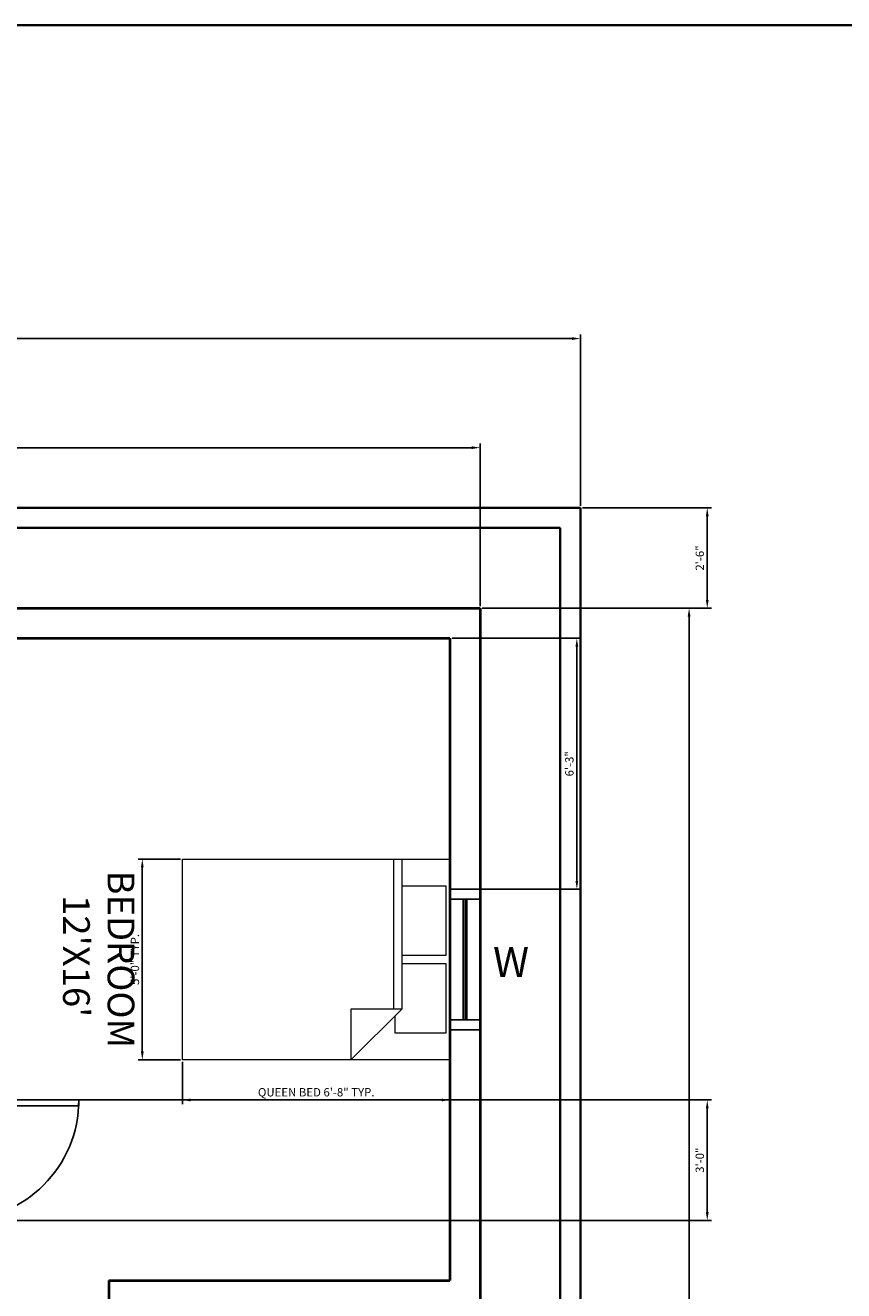
# Model space of a CAD drawing. Units: inches. Extents: x 6038 to 7543, y 3772 to 5131.
# Tile 9 of 14: x 6545 to 6790, y 4753 to 5131. Entities that reach past the tile are written whole.
import ezdxf

# ---------------------------------------------------------------- set-up
doc = ezdxf.new("R2010")
doc.units = ezdxf.units.IN
for name, color, linetype, lineweight in [('A-ANNO-DIMS', 4, 'Continuous', 18), ('A-ANNO-TEXT', 7, 'Continuous', 18), ('A-ANNO-TTLB', 1, 'Continuous', 35), ('A-AREA-IDEN', 2, 'Continuous', 18), ('A-DOOR', 3, 'Continuous', 25), ('A-FURN', 8, 'Continuous', 18), ('A-WALL', 7, 'Continuous', 40)]:
    doc.layers.add(name, color=color, linetype=linetype, lineweight=lineweight)
doc.layers.add('A-GLAZ', color=30, linetype='Continuous', lineweight=25, true_color=0xf26722)
doc.layers.add('C-PROP-WALL', color=251, linetype='Continuous', lineweight=35, true_color=0x636466)
doc.styles.get("Standard").update_dxf_attribs({"font": 'arial.ttf'})
doc.dimstyles.new('ISO-25', dxfattribs={"dimtxt": 2.5, "dimasz": 2.5, "dimexe": 1.25, "dimexo": 0.625, "dimtad": 1, "dimdec": 0, "dimlunit": 3, "dimtxsty": 'Standard', "dimcen": 2.5, "dimadec": 0, "dimazin": 0, "dimtfac": 1, "dimtdec": 0, "dimtmove": 0, "dimatfit": 3, "dimfxl": 1, "dimarcsym": 0})

# ---------------------------------------------------------------- blocks, each defined once
blk = doc.blocks.new('Bed - Queen')
for p, q in [((0, -80.00003), (0, 0)), ((0, 0), (59.99999, 0)), ((59.99999, 0), (59.99999, -80.00003)), ((7.99999, -1.2), (28.79998, -1.2)), ((7.99999, -14.4), (7.99999, -1.2)), ((28.79998, -1.2), (28.79998, -14.4)), ((31.19999, -1.2), (51.99999, -1.2)), ((31.19999, -14.4), (31.19999, -1.2)), ((51.99999, -1.2), (51.99999, -16.4)), ((0, -14.4), (44.8, -14.4)), ((59.99999, -29.6), (44.8, -14.4)), ((44.8, -14.4), (44.8, -29.6)), ((44.8, -16.8), (0, -16.8)), ((51.99999, -16.4), (46.79936, -16.4)), ((44.8, -29.6), (59.99999, -29.6)), ((59.99999, -80.00003), (0, -80.00003))]:
    blk.add_line(p, q)
blk = doc.blocks.new('*U9')
for p, q in [((0, 0), (0, -6)), ((36, 0), (36, -6))]:
    blk.add_line(p, q)
blk.add_lwpolyline([(0, 0), (0, 36), (1.75, 36), (1.75, 0)], close=True)
blk.add_arc((0, 0), 36, 0, 90)
blk = doc.blocks.new('*D13')
at = {"layer": 'A-ANNO-DIMS', "color": 0, "lineweight": -2, "transparency": 16777216}
for p, q in [((6321.42, 4957.24), (6321.42, 5005.85)), ((6323.92, 5004.6), (6678.92, 5004.6)), ((6681.42, 4957.24), (6681.42, 5005.85))]:
    blk.add_line(p, q, dxfattribs=at)
at = {"layer": 'A-ANNO-DIMS', "color": 0, "transparency": 16777216}
for points in [[(6323.92, 5005.02), (6323.92, 5004.19), (6321.42, 5004.6)], [(6678.92, 5005.02), (6678.92, 5004.19), (6681.42, 5004.6)]]:
    blk.add_solid(points, dxfattribs=at)
at = {"layer": 'Defpoints', "color": 0, "transparency": 16777216}
for p in [(6681.42, 5004.6), (6321.42, 4956.62), (6681.42, 4956.62)]:
    blk.add_point(p, dxfattribs=at)
at = {"layer": 'A-ANNO-DIMS', "color": 0, "transparency": 16777216, "insert": (6501.42, 5012.89), "char_height": 2.5, "attachment_point": 5}
blk.add_mtext("{\\H6x;30'}", dxfattribs=at)
blk = doc.blocks.new('*D14')
at = {"layer": 'A-ANNO-DIMS', "color": 0, "lineweight": -2, "transparency": 16777216}
for p, q in [((6682.04, 4956.62), (6745.18, 4956.62)), ((6743.93, 4954.12), (6743.93, 4371.12)), ((6682.04, 4368.62), (6745.18, 4368.62))]:
    blk.add_line(p, q, dxfattribs=at)
at = {"layer": 'A-ANNO-DIMS', "color": 0, "transparency": 16777216}
for points in [[(6743.51, 4954.12), (6744.35, 4954.12), (6743.93, 4956.62)], [(6743.51, 4371.12), (6744.35, 4371.12), (6743.93, 4368.62)]]:
    blk.add_solid(points, dxfattribs=at)
at = {"layer": 'Defpoints', "color": 0, "transparency": 16777216}
for p in [(6681.42, 4956.62), (6681.42, 4368.62), (6743.93, 4368.62)]:
    blk.add_point(p, dxfattribs=at)
at = {"layer": 'A-ANNO-DIMS', "color": 0, "transparency": 16777216, "insert": (6735.65, 4662.62), "char_height": 2.5, "attachment_point": 5, "rotation": 90}
blk.add_mtext("{\\H6x;49'}", dxfattribs=at)
blk = doc.blocks.new('*D16')
at = {"layer": 'A-ANNO-DIMS', "color": 0, "lineweight": -2, "transparency": 16777216}
for p, q in [((6291.42, 4987.24), (6291.42, 5038.47)), ((6711.42, 4987.24), (6711.42, 5038.47)), ((6293.92, 5037.22), (6708.92, 5037.22))]:
    blk.add_line(p, q, dxfattribs=at)
at = {"layer": 'A-ANNO-DIMS', "color": 0, "transparency": 16777216}
for points in [[(6293.92, 5037.63), (6293.92, 5036.8), (6291.42, 5037.22)], [(6708.92, 5037.63), (6708.92, 5036.8), (6711.42, 5037.22)]]:
    blk.add_solid(points, dxfattribs=at)
at = {"layer": 'Defpoints', "color": 0, "transparency": 16777216}
for p in [(6711.42, 5037.22), (6291.42, 4986.62), (6711.42, 4986.62)]:
    blk.add_point(p, dxfattribs=at)
at = {"layer": 'A-ANNO-DIMS', "color": 0, "transparency": 16777216, "insert": (6501.42, 5046.53), "char_height": 2.5, "attachment_point": 5}
blk.add_mtext("{\\H6.8x;35'}", dxfattribs=at)
blk = doc.blocks.new('WIN-36-PLAN')
for p, q in [((9, 42), (0, 42)), ((9, 39), (0, 39)), ((4, 39), (4, 3)), ((4.5, 39), (4.5, 3)), ((5, 39), (5, 3)), ((9, 3), (0, 3)), ((9, 0), (0, 0))]:
    blk.add_line(p, q)
blk = doc.blocks.new('*D36')
at = {"layer": 'A-ANNO-DIMS', "color": 0, "lineweight": -2, "transparency": 16777216}
for p, q in [((6592.42, 4820.99), (6592.42, 4808.37)), ((6672.42, 4820.99), (6672.42, 4808.37)), ((6594.92, 4809.62), (6669.92, 4809.62))]:
    blk.add_line(p, q, dxfattribs=at)
at = {"layer": 'A-ANNO-DIMS', "color": 0, "transparency": 16777216}
for points in [[(6594.92, 4810.04), (6594.92, 4809.2), (6592.42, 4809.62)], [(6669.92, 4810.04), (6669.92, 4809.2), (6672.42, 4809.62)]]:
    blk.add_solid(points, dxfattribs=at)
at = {"layer": 'Defpoints', "color": 0, "transparency": 16777216}
for p in [(6592.42, 4821.62), (6672.42, 4821.62), (6672.42, 4809.62)]:
    blk.add_point(p, dxfattribs=at)
at = {"layer": 'A-ANNO-DIMS', "color": 0, "transparency": 16777216, "insert": (6632.42, 4811.61), "char_height": 2.5, "attachment_point": 5}
blk.add_mtext('QUEEN BED 6\'-8" TYP.', dxfattribs=at)
blk = doc.blocks.new('*D37')
at = {"layer": 'A-ANNO-DIMS', "color": 0, "lineweight": -2, "transparency": 16777216}
for p, q in [((6591.79, 4881.62), (6579.17, 4881.62)), ((6580.42, 4879.12), (6580.42, 4824.12)), ((6591.79, 4821.62), (6579.17, 4821.62))]:
    blk.add_line(p, q, dxfattribs=at)
at = {"layer": 'A-ANNO-DIMS', "color": 0, "transparency": 16777216}
for points in [[(6580, 4879.12), (6580.83, 4879.12), (6580.42, 4881.62)], [(6580, 4824.12), (6580.83, 4824.12), (6580.42, 4821.62)]]:
    blk.add_solid(points, dxfattribs=at)
at = {"layer": 'Defpoints', "color": 0, "transparency": 16777216}
for p in [(6592.42, 4881.62), (6580.42, 4821.62), (6592.42, 4821.62)]:
    blk.add_point(p, dxfattribs=at)
at = {"layer": 'A-ANNO-DIMS', "color": 0, "transparency": 16777216, "insert": (6578.52, 4851.62), "char_height": 2.5, "attachment_point": 5, "rotation": 90}
blk.add_mtext('5\'-0" TYP.', dxfattribs=at)
blk = doc.blocks.new('*D55')
at = {"layer": 'A-ANNO-DIMS', "color": 0, "lineweight": -2, "transparency": 16777216}
for p, q in [((6712.04, 4986.62), (6750.62, 4986.62)), ((6749.37, 4984.12), (6749.37, 4959.12)), ((6682.04, 4956.62), (6750.62, 4956.62))]:
    blk.add_line(p, q, dxfattribs=at)
at = {"layer": 'A-ANNO-DIMS', "color": 0, "transparency": 16777216}
for points in [[(6748.95, 4984.12), (6749.78, 4984.12), (6749.37, 4986.62)], [(6748.95, 4959.12), (6749.78, 4959.12), (6749.37, 4956.62)]]:
    blk.add_solid(points, dxfattribs=at)
at = {"layer": 'Defpoints', "color": 0, "transparency": 16777216}
for p in [(6711.42, 4986.62), (6681.42, 4956.62), (6749.37, 4956.62)]:
    blk.add_point(p, dxfattribs=at)
at = {"layer": 'A-ANNO-DIMS', "color": 0, "transparency": 16777216, "insert": (6747.47, 4971.62), "char_height": 2.5, "attachment_point": 5, "rotation": 90}
blk.add_mtext('2\'-6"', dxfattribs=at)
blk = doc.blocks.new('*D58')
at = {"layer": 'A-ANNO-DIMS', "color": 0, "lineweight": -2, "transparency": 16777216}
for p, q in [((6520.04, 4809.62), (6750.62, 4809.62)), ((6749.37, 4807.12), (6749.37, 4776.12)), ((6520.04, 4773.62), (6750.62, 4773.62))]:
    blk.add_line(p, q, dxfattribs=at)
at = {"layer": 'A-ANNO-DIMS', "color": 0, "transparency": 16777216}
for points in [[(6748.95, 4807.12), (6749.78, 4807.12), (6749.37, 4809.62)], [(6748.95, 4776.12), (6749.78, 4776.12), (6749.37, 4773.62)]]:
    blk.add_solid(points, dxfattribs=at)
at = {"layer": 'Defpoints', "color": 0, "transparency": 16777216}
for p in [(6519.42, 4809.62), (6519.42, 4773.62), (6749.37, 4773.62)]:
    blk.add_point(p, dxfattribs=at)
at = {"layer": 'A-ANNO-DIMS', "color": 0, "transparency": 16777216, "insert": (6747.46, 4791.62), "char_height": 2.5, "attachment_point": 5, "rotation": 90}
blk.add_mtext('3\'-0"', dxfattribs=at)
blk = doc.blocks.new('*D60')
at = {"layer": 'A-ANNO-DIMS', "color": 0, "lineweight": -2, "transparency": 16777216}
for p, q in [((6673.04, 4947.62), (6711.62, 4947.62)), ((6710.37, 4945.12), (6710.37, 4875.12)), ((6673.04, 4872.62), (6711.62, 4872.62))]:
    blk.add_line(p, q, dxfattribs=at)
at = {"layer": 'A-ANNO-DIMS', "color": 0, "transparency": 16777216}
for points in [[(6709.95, 4945.12), (6710.78, 4945.12), (6710.37, 4947.62)], [(6709.95, 4875.12), (6710.78, 4875.12), (6710.37, 4872.62)]]:
    blk.add_solid(points, dxfattribs=at)
at = {"layer": 'Defpoints', "color": 0, "transparency": 16777216}
for p in [(6672.42, 4947.62), (6672.42, 4872.62), (6710.37, 4872.62)]:
    blk.add_point(p, dxfattribs=at)
at = {"layer": 'A-ANNO-DIMS', "color": 0, "transparency": 16777216, "insert": (6708.46, 4910.12), "char_height": 2.5, "attachment_point": 5, "rotation": 90}
blk.add_mtext('6\'-3"', dxfattribs=at)

msp = doc.modelspace()

# ---------------------------------------------------------------- linework, layer by layer
at = {"layer": 'A-ANNO-TTLB'}
msp.add_lwpolyline([(6037.83, 5130.86), (7542.53, 5130.86), (7542.53, 3772.09), (6037.83, 3772.09)], close=True, dxfattribs=at)
at = {"layer": 'A-WALL'}
for p, q in [((6321.42, 4956.62), (6681.42, 4956.62)), ((6681.42, 4956.62), (6681.42, 4368.62)), ((6528.42, 4947.62), (6672.42, 4947.62)), ((6672.42, 4947.62), (6672.42, 4755.62)), ((6570.42, 4755.62), (6570.42, 4749.62)), ((6570.42, 4755.62), (6672.42, 4755.62))]:
    msp.add_line(p, q, dxfattribs=at)
at = {"layer": 'C-PROP-WALL'}
for p, q in [((6291.42, 4986.62), (6711.42, 4986.62)), ((6711.42, 4986.62), (6711.42, 4362.62)), ((6297.42, 4980.62), (6705.42, 4980.62)), ((6705.42, 4980.62), (6705.42, 4368.62))]:
    msp.add_line(p, q, dxfattribs=at)

# ---------------------------------------------------------------- block references
at = {"layer": 'A-DOOR', "rotation": 270}
msp.add_blockref('*U9', (6525.42, 4809.62), dxfattribs=at)
at = {"layer": 'A-FURN', "rotation": 270}
msp.add_blockref('Bed - Queen', (6672.42, 4881.62), dxfattribs=at)
at = {"layer": 'A-GLAZ'}
msp.add_blockref('WIN-36-PLAN', (6672.42, 4830.62), dxfattribs=at)

# ---------------------------------------------------------------- texts
at = {"layer": 'A-ANNO-TEXT', "insert": (6685.3, 4855.38), "char_height": 9, "attachment_point": 1}
msp.add_mtext_dynamic_manual_height_columns('W', width=212.1416, gutter_width=12.5, heights=[0], dxfattribs=at)
at = {"layer": 'A-AREA-IDEN', "insert": (6578.04, 4878.22), "char_height": 8, "attachment_point": 1, "rotation": 270}
msp.add_mtext_dynamic_manual_height_columns("BEDROOM\\P   12'X16'", width=589.9095, gutter_width=12.5, heights=[0], dxfattribs=at)

# ---------------------------------------------------------------- dimensions: what is measured, and where the dimension line sits
at = {"layer": 'A-ANNO-DIMS'}
for base, p1, p2, text, override, picture, middle in [((6711.42, 5037.22), (6291.42, 4986.62), (6711.42, 4986.62), '{\\H6.8x;<>}', {"dimclrd": 0, "dimclre": 0, "dimclrt": 0}, '*D16', (6501.42, 5046.53)), ((6681.42, 5004.6), (6321.42, 4956.62), (6681.42, 4956.62), '{\\H6x;<>}', {"dimclrd": 0, "dimclre": 0, "dimclrt": 0}, '*D13', (6501.42, 5012.89)), ((6672.42, 4809.62), (6592.42, 4821.62), (6672.42, 4821.62), 'QUEEN BED <> TYP.', {"dimdec": 1, "dimlfac": 1, "dimrnd": 0, "dimzin": 1, "dimdsep": 46, "dimlunit": 4, "dimfrac": 2}, '*D36', (6632.42, 4811.61))]:
    dim = msp.add_linear_dim(base=base, p1=p1, p2=p2, text=text, dimstyle='ISO-25', override=override, dxfattribs=at)
    dim.commit()
    dim.dimension.update_dxf_attribs({"geometry": picture, "text_midpoint": middle})
for base, p1, p2, angle, picture, middle in [((6749.37, 4956.62), (6711.42, 4986.62), (6681.42, 4956.62), 90, '*D55', (6747.47, 4971.62)), ((6710.37, 4872.62), (6672.42, 4947.62), (6672.42, 4872.62), 270, '*D60', (6708.46, 4910.12)), ((6749.37, 4773.62), (6519.42, 4809.62), (6519.42, 4773.62), 90, '*D58', (6747.46, 4791.62))]:
    dim = msp.add_linear_dim(base=base, p1=p1, p2=p2, angle=angle, dimstyle='ISO-25', override={"dimdec": 1, "dimlfac": 1, "dimrnd": 0, "dimzin": 1, "dimdsep": 46, "dimlunit": 4, "dimfrac": 2}, dxfattribs=at)
    dim.commit()
    dim.dimension.update_dxf_attribs({"geometry": picture, "text_midpoint": middle})
for base, p1, p2, angle, text, override, picture, middle in [((6743.93, 4368.62), (6681.42, 4956.62), (6681.42, 4368.62), 90, '{\\H6x;<>}', {"dimclrd": 0, "dimclre": 0, "dimclrt": 0}, '*D14', (6735.65, 4662.62)), ((6580.42, 4821.62), (6592.42, 4881.62), (6592.42, 4821.62), 270, '<> TYP.', {"dimdec": 1, "dimlfac": 1, "dimrnd": 0, "dimzin": 1, "dimdsep": 46, "dimlunit": 4, "dimfrac": 2}, '*D37', (6578.52, 4851.62))]:
    dim = msp.add_linear_dim(base=base, p1=p1, p2=p2, angle=angle, text=text, dimstyle='ISO-25', override=override, dxfattribs=at)
    dim.commit()
    dim.dimension.update_dxf_attribs({"geometry": picture, "text_midpoint": middle})

doc.saveas('drawing.dxf')
